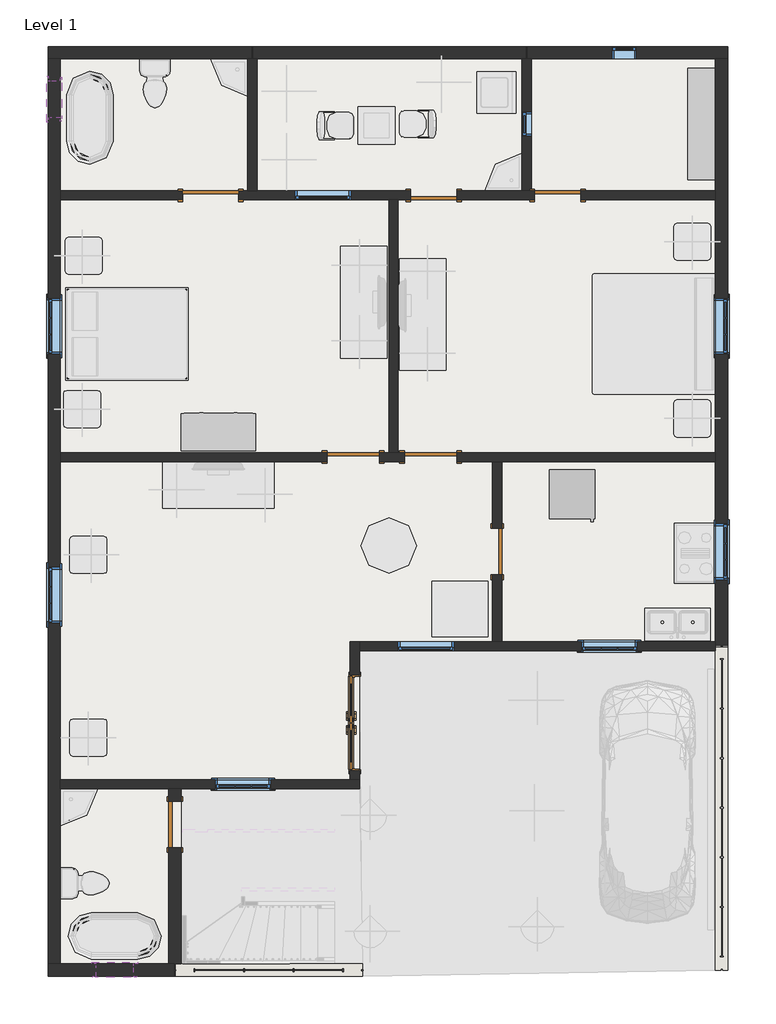
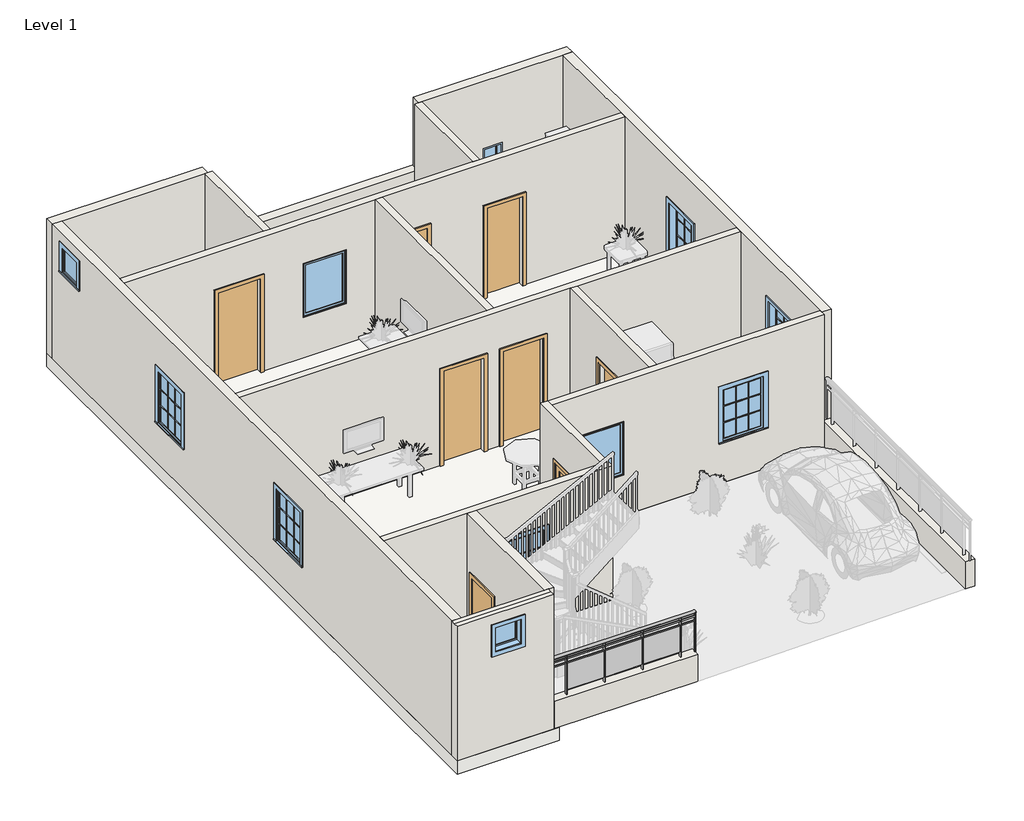
# One storey, part 1 of 3: 18 walls, 12 windows, 8 doors, 1 railing, 1 slab.
"""IFC4 building model written with IfcOpenShell, lengths in millimetres."""

from ifc_helpers import new_model, si_unit, point, frame, origin, origin_with_axes, place, context, project, spatial, polyline, ellipse_curve, trimmed, outline, extrude, faceted_brep, transform, mapped, element, save
from ifc_brep_helpers import plane_surface, extruded_surface, advanced_brep
from components import door_94998e6c, door_059fdd7e, door_255cab33, door_d8ec59b1, door_b6e9fca3, door_99d96fc5, door_16372e1c, window_29c06734, window_5c190c7e, window_7ecdf1d7, window_085f26e1, window_d657a5cb, window_e41d21a6

model = new_model("IFC4")

# Units and contexts
model_context = context("Model", 3, world=origin())
ifc_project = project(units=[si_unit("LENGTHUNIT", "METRE", prefix="MILLI")], contexts=[model_context])

# Site, building, storey
site = spatial("IfcSite", under=ifc_project)
building = spatial("IfcBuilding", under=site)
storey = spatial("IfcBuildingStorey", under=building, Name="Level 1", Elevation=0.0)

# Doors
placement = place(None, origin())
door_shape = door_94998e6c(model_context)
element("IfcDoor", 1, ObjectType="Door-Exterior-Double-Full Glass-Wood_Clad : 60\" x 80\"", at=placement, inside=storey, context=model_context, shape_type="MappedRepresentation", body=[
    mapped(door_shape, transform((-7732.5242777, 3282.853629, 0.0), x_axis=(0.0, 1.0, 0.0), y_axis=(-1.0, 0.0, 0.0), z_axis=(0.0, 0.0, 1.0))),
])
door_2_shape = door_059fdd7e(model_context)
element("IfcDoor", 2, ObjectType="Single-Flush : 30\" x 80\"", at=placement, inside=storey, context=model_context, shape_type="MappedRepresentation", body=[
    mapped(door_2_shape, transform((-6433.9492777, 11931.553629, 0.0), x_axis=(-1.0, 0.0, 0.0), y_axis=(0.0, -1.0, 0.0), z_axis=(0.0, 0.0, 1.0))),
])
element("IfcDoor", 3, ObjectType="Single-Flush : 30\" x 80\"", at=placement, inside=storey, context=model_context, shape_type="MappedRepresentation", body=[
    mapped(door_2_shape, transform((-5392.5492777, 6089.553629, 0.0), x_axis=(0.0, -1.0, 0.0), y_axis=(1.0, 0.0, 0.0), z_axis=(0.0, 0.0, 1.0))),
])
door_3_shape = door_255cab33(model_context)
element("IfcDoor", 4, ObjectType="Single-Flush : 30\" x 80\"", at=placement, inside=storey, context=model_context, shape_type="MappedRepresentation", body=[
    mapped(door_3_shape, transform((-4401.9492777, 11931.553629, 0.0), x_axis=(-1.0, 0.0, 0.0), y_axis=(0.0, -1.0, 0.0), z_axis=(0.0, 0.0, 1.0))),
])
door_4_shape = door_d8ec59b1(model_context)
element("IfcDoor", 5, ObjectType="Single-Flush : 30\" x 80\" 2", at=placement, inside=storey, context=model_context, shape_type="MappedRepresentation", body=[
    mapped(door_4_shape, transform((-10675.7492777, 1619.153629, 0.0), x_axis=(0.0, 1.0, 0.0), y_axis=(-1.0, 0.0, 0.0), z_axis=(0.0, 0.0, 1.0))),
])
door_5_shape = door_b6e9fca3(model_context)
element("IfcDoor", 6, ObjectType="Single-Flush : 34\" x 84\"", at=placement, inside=storey, context=model_context, shape_type="MappedRepresentation", body=[
    mapped(door_5_shape, transform((-7754.7492777, 7638.953629, 0.0), x_axis=(1.0, 0.0, 0.0), y_axis=(0.0, 1.0, 0.0), z_axis=(0.0, 0.0, 1.0))),
])
door_6_shape = door_99d96fc5(model_context)
element("IfcDoor", 7, ObjectType="Single-Flush : 34\" x 84\"", at=placement, inside=storey, context=model_context, shape_type="MappedRepresentation", body=[
    mapped(door_6_shape, transform((-6484.7492777, 7638.953629, 0.0), x_axis=(-1.0, 0.0, 0.0), y_axis=(0.0, -1.0, 0.0), z_axis=(0.0, 0.0, 1.0))),
])
door_7_shape = door_16372e1c(model_context)
element("IfcDoor", 8, ObjectType="Single-Flush : 36\" x 84\"", at=placement, inside=storey, context=model_context, shape_type="MappedRepresentation", body=[
    mapped(door_7_shape, transform((-10091.5492777, 11931.553629, 0.0), x_axis=(1.0, 0.0, 0.0), y_axis=(0.0, 1.0, 0.0), z_axis=(0.0, 0.0, 1.0))),
])

# Railing
element("IfcRailing", 9, ObjectType="Glass Panel - Bottom Fill", at=placement, inside=storey, context=model_context, shape_type="SolidModel", body=[
    advanced_brep(
    [(-10675.7492777, -730.346371, 1524.0), (-10675.7492777, -806.546371, 1524.0), (-7602.3492777, -730.346371, 1524.0), (-7602.3492777, -806.546371, 1524.0)],
    [
        (0, 1, ellipse_curve(frame((-10675.7492777, -768.446371, 1524.0), z_axis=(-1.0, 0.0, 0.0), x_axis=(0.0, -1.0, 0.0)), 38.1, 28.575)),
        (1, 0, ellipse_curve(frame((-10675.7492777, -768.446371, 1524.0), z_axis=(-1.0, 0.0, 0.0), x_axis=(0.0, -1.0, 0.0)), 38.1, 28.575)),
        (2, 3, ellipse_curve(frame((-7602.3492777, -768.446371, 1524.0), z_axis=(1.0, 0.0, 0.0), x_axis=(0.0, -1.0, 0.0)), 38.1, 28.575)),
        (3, 2, ellipse_curve(frame((-7602.3492777, -768.446371, 1524.0), z_axis=(1.0, 0.0, 0.0), x_axis=(0.0, -1.0, 0.0)), 38.1, 28.575)),
        (0, 2),
        (3, 1),
    ],
    [
        plane_surface(frame((-10675.7492777, -768.446371, 1524.0), z_axis=(-1.0, 0.0, 0.0), x_axis=(0.0, 1.0, 0.0))),
        plane_surface(frame((-7602.3492777, -768.446371, 1524.0), z_axis=(1.0, 0.0, 0.0), x_axis=(0.0, 1.0, 0.0))),
        extruded_surface(trimmed(ellipse_curve(frame((-7602.3492777, -768.446371, 1524.0), z_axis=(-1.0, 0.0, 0.0), x_axis=(0.0, -1.0, 0.0)), 38.1, 28.575), [point((-7602.3492777, -730.346371, 1524.0))], [point((-7602.3492777, -806.546371, 1524.0))], True, "CARTESIAN"), (-3073.4000000000005, 0.0, 0.0), 3073.4000000000005),
        extruded_surface(trimmed(ellipse_curve(frame((-7602.3492777, -768.446371, 1524.0), z_axis=(-1.0, 0.0, 0.0), x_axis=(0.0, -1.0, 0.0)), 38.1, 28.575), [point((-7602.3492777, -806.546371, 1524.0))], [point((-7602.3492777, -730.346371, 1524.0))], True, "CARTESIAN"), (-3073.4000000000005, 0.0, 0.0), 3073.4000000000005),
    ],
    [
        (0, [[1, 2]]),
        (1, [[3, 4]]),
        (2, [[-1, 5, -4, 6]]),
        (3, [[-2, -6, -3, -5]]),
    ],
),
    extrude(outline(polyline([(-10675.7492777, -781.146371), (-10675.7492777, -755.746371), (-7602.3492777, -755.746371), (-7602.3492777, -781.146371), (-10675.7492777, -781.146371)])), frame((0.0, 0.0, 1409.7), z_axis=(0.0, 0.0, 1.0), x_axis=(1.0, 0.0, 0.0)), (0.0, 0.0, 1.0), 25.4),
    extrude(outline(polyline([(-10675.7492777, -781.146371), (-10675.7492777, -755.746371), (-7602.3492777, -755.746371), (-7602.3492777, -781.146371), (-10675.7492777, -781.146371)])), frame((0.0, 0.0, 1308.1), z_axis=(0.0, 0.0, 1.0), x_axis=(1.0, 0.0, 0.0)), (0.0, 0.0, 1.0), 25.4),
    extrude(outline(polyline([(-7926.1992777, -793.846371), (-7926.1992777, -743.046371), (-7913.4992777, -743.046371), (-7913.4992777, -793.846371), (-7926.1992777, -793.846371)])), frame((0.0, 0.0, 609.6), z_axis=(0.0, 0.0, 1.0), x_axis=(1.0, 0.0, 0.0)), (0.0, 0.0, 1.0), 885.6788223),
    extrude(outline(polyline([(-8732.6492777, -761.911214), (-7919.8492777, -761.911214), (-7919.8492777, -768.261214), (-8732.6492777, -768.261214), (-8732.6492777, -761.911214)])), frame((0.0, 0.0, 711.2), z_axis=(0.0, 0.0, 1.0), x_axis=(1.0, 0.0, 0.0)), (0.0, 0.0, 1.0), 596.9),
    extrude(outline(polyline([(-8738.9992777, -793.846371), (-8738.9992777, -743.046371), (-8726.2992777, -743.046371), (-8726.2992777, -793.846371), (-8738.9992777, -793.846371)])), frame((0.0, 0.0, 609.6), z_axis=(0.0, 0.0, 1.0), x_axis=(1.0, 0.0, 0.0)), (0.0, 0.0, 1.0), 885.6788223),
    extrude(outline(polyline([(-9545.4492777, -761.911214), (-8732.6492777, -761.911214), (-8732.6492777, -768.261214), (-9545.4492777, -768.261214), (-9545.4492777, -761.911214)])), frame((0.0, 0.0, 711.2), z_axis=(0.0, 0.0, 1.0), x_axis=(1.0, 0.0, 0.0)), (0.0, 0.0, 1.0), 596.9),
    extrude(outline(polyline([(-9551.7992777, -793.846371), (-9551.7992777, -743.046371), (-9539.0992777, -743.046371), (-9539.0992777, -793.846371), (-9551.7992777, -793.846371)])), frame((0.0, 0.0, 609.6), z_axis=(0.0, 0.0, 1.0), x_axis=(1.0, 0.0, 0.0)), (0.0, 0.0, 1.0), 885.6788223),
    extrude(outline(polyline([(-10358.2492777, -761.911214), (-9545.4492777, -761.911214), (-9545.4492777, -768.261214), (-10358.2492777, -768.261214), (-10358.2492777, -761.911214)])), frame((0.0, 0.0, 711.2), z_axis=(0.0, 0.0, 1.0), x_axis=(1.0, 0.0, 0.0)), (0.0, 0.0, 1.0), 596.9),
    extrude(outline(polyline([(-10364.5992777, -793.846371), (-10364.5992777, -743.046371), (-10351.8992777, -743.046371), (-10351.8992777, -793.846371), (-10364.5992777, -793.846371)])), frame((0.0, 0.0, 609.6), z_axis=(0.0, 0.0, 1.0), x_axis=(1.0, 0.0, 0.0)), (0.0, 0.0, 1.0), 885.6788223),
    extrude(outline(polyline([(-7615.0492777, -777.971371), (-7615.0492777, -758.921371), (-7595.9992777, -758.921371), (-7595.9992777, -777.971371), (-7615.0492777, -777.971371)])), frame((0.0, 0.0, 609.6), z_axis=(0.0, 0.0, 1.0), x_axis=(1.0, 0.0, 0.0)), (0.0, 0.0, 1.0), 885.6788223),
    extrude(outline(polyline([(-10682.0992777, -777.971371), (-10682.0992777, -758.921371), (-10663.0492777, -758.921371), (-10663.0492777, -777.971371), (-10682.0992777, -777.971371)])), frame((0.0, 0.0, 609.6), z_axis=(0.0, 0.0, 1.0), x_axis=(1.0, 0.0, 0.0)), (0.0, 0.0, 1.0), 885.6788223),
])

# Slab
element("IfcSlab", 10, ObjectType="Generic - 12\"", at=placement, inside=storey, context=model_context, shape_type="SweptSolid", body=[
    extrude(outline(polyline([(-1607.9492777, 14369.953629), (-1607.9492777, 4463.953629), (-7653.1492777, 4463.953629), (-7653.1492777, 2203.353629), (-10574.1492777, 2203.353629), (-10574.1492777, -870.046371), (-12758.5492777, -870.046371), (-12758.5492777, 14369.953629), (-1607.9492777, 14369.953629)])), frame((0.0, 0.0, -304.8), z_axis=(0.0, 0.0, 1.0), x_axis=(1.0, 0.0, 0.0)), (0.0, 0.0, 1.0), 304.8),
])

# Walls
element("IfcWall", 11, ObjectType="Generic - 2'", at=placement, inside=storey, context=model_context, shape_type="Brep", body=[
    faceted_brep([(-1811.1492777, 4527.453629, 0.0), (-1811.1492777, 4463.953629, 0.0), (-1811.1492777, -768.446371, 0.0), (-1811.1492777, -768.446371, 609.6), (-1811.1492777, 4527.453629, 609.6), (-1607.9492777, 4527.453629, 0.0), (-1607.9492777, 4527.453629, 609.6), (-1607.9492777, -768.446371, 609.6), (-1607.9492777, -768.446371, 0.0)], [[[0, 1, 2, 3, 4]], [[5, 6, 7, 8]], [[2, 1, 0, 5, 8]], [[3, 2, 8, 7]], [[4, 3, 7, 6]], [[0, 4, 6, 5]]]),
])
element("IfcWall", 12, ObjectType="Generic - 2'", at=placement, inside=storey, context=model_context, shape_type="SweptSolid", body=[
    extrude(outline(polyline([(-10663.0492777, -666.846371), (-7602.3492777, -666.846371), (-7602.3492777, -870.046371), (-10663.0492777, -870.046371), (-10663.0492777, -666.846371)])), origin_with_axes(), (0.0, 0.0, 1.0), 609.6),
])
element("IfcWall", 13, ObjectType="Generic - 8\"", at=placement, inside=storey, context=model_context, shape_type="Brep", body=[
    faceted_brep([(-12758.5492777, 14166.753629, 0.0), (-12555.3492777, 14166.753629, 0.0), (-9418.4492777, 14166.753629, 0.0), (-9418.4492777, 14166.753629, 3048.0), (-12555.3492777, 14166.753629, 3048.0), (-12758.5492777, 14166.753629, 3048.0), (-12758.5492777, 14369.953629, 0.0), (-12758.5492777, 14369.953629, 3048.0), (-9418.4492777, 14369.953629, 3048.0), (-9418.4492777, 14369.953629, 0.0)], [[[0, 1, 2, 3, 4, 5]], [[6, 7, 8, 9]], [[2, 1, 0, 6, 9]], [[3, 2, 9, 8]], [[0, 5, 7, 6]], [[5, 4, 3, 8, 7]]]),
])
element("IfcWall", 14, ObjectType="Generic - 8\"", at=placement, inside=storey, context=model_context, shape_type="Brep", body=[
    faceted_brep([(-1811.1492777, 14166.753629, 0.0), (-1811.1492777, 12007.753629, 0.0), (-1811.1492777, 11855.353629, 0.0), (-1811.1492777, 7715.153629, 0.0), (-1811.1492777, 7562.753629, 0.0), (-1811.1492777, 4552.853629, 0.0), (-1811.1492777, 4552.853629, 3048.0), (-1811.1492777, 7562.753629, 3048.0), (-1811.1492777, 7715.153629, 3048.0), (-1811.1492777, 11855.353629, 3048.0), (-1811.1492777, 12007.753629, 3048.0), (-1811.1492777, 14166.753629, 3048.0), (-1811.1492777, 9328.053629, 2133.6), (-1811.1492777, 9328.053629, 914.4), (-1811.1492777, 10242.453629, 914.4), (-1811.1492777, 10242.453629, 2133.6), (-1811.1492777, 5632.353629, 2133.6), (-1811.1492777, 5632.353629, 914.4), (-1811.1492777, 6546.753629, 914.4), (-1811.1492777, 6546.753629, 2133.6), (-1607.9492777, 14166.753629, 0.0), (-1607.9492777, 14166.753629, 3048.0), (-1607.9492777, 4552.853629, 3048.0), (-1607.9492777, 4552.853629, 0.0), (-1607.9492777, 9328.053629, 2133.6), (-1607.9492777, 10242.453629, 2133.6), (-1607.9492777, 10242.453629, 914.4), (-1607.9492777, 9328.053629, 914.4), (-1607.9492777, 5632.353629, 2133.6), (-1607.9492777, 6546.753629, 2133.6), (-1607.9492777, 6546.753629, 914.4), (-1607.9492777, 5632.353629, 914.4)], [[[0, 1, 2, 3, 4, 5, 6, 7, 8, 9, 10, 11], [12, 13, 14, 15], [16, 17, 18, 19]], [[20, 21, 22, 23], [24, 25, 26, 27], [28, 29, 30, 31]], [[5, 4, 3, 2, 1, 0, 20, 23]], [[6, 5, 23, 22]], [[0, 11, 21, 20]], [[13, 12, 24, 27]], [[14, 13, 27, 26]], [[15, 14, 26, 25]], [[12, 15, 25, 24]], [[17, 16, 28, 31]], [[18, 17, 31, 30]], [[19, 18, 30, 29]], [[16, 19, 29, 28]], [[11, 10, 9, 8, 7, 6, 22, 21]]]),
])
element("IfcWall", 15, ObjectType="Generic - 8\"", at=placement, inside=storey, context=model_context, shape_type="Brep", body=[
    faceted_brep([(-12555.3492777, -666.846371, 0.0), (-12555.3492777, 2203.353629, 0.0), (-12555.3492777, 2355.753629, 0.0), (-12555.3492777, 7562.753629, 0.0), (-12555.3492777, 7715.153629, 0.0), (-12555.3492777, 11855.353629, 0.0), (-12555.3492777, 12007.753629, 0.0), (-12555.3492777, 14166.753629, 0.0), (-12555.3492777, 14166.753629, 3048.0), (-12555.3492777, 12007.753629, 3048.0), (-12555.3492777, 11855.353629, 3048.0), (-12555.3492777, 7715.153629, 3048.0), (-12555.3492777, 7562.753629, 3048.0), (-12555.3492777, 2355.753629, 3048.0), (-12555.3492777, 2203.353629, 3048.0), (-12555.3492777, -666.846371, 3048.0), (-12555.3492777, 13811.153629, 2768.6), (-12555.3492777, 13811.153629, 2159.0), (-12555.3492777, 13201.553629, 2159.0), (-12555.3492777, 13201.553629, 2768.6), (-12555.3492777, 10242.453629, 2133.6), (-12555.3492777, 10242.453629, 914.4), (-12555.3492777, 9328.053629, 914.4), (-12555.3492777, 9328.053629, 2133.6), (-12555.3492777, 5835.553629, 2133.6), (-12555.3492777, 5835.553629, 914.4), (-12555.3492777, 4921.153629, 914.4), (-12555.3492777, 4921.153629, 2133.6), (-12758.5492777, -666.846371, 0.0), (-12758.5492777, -666.846371, 3048.0), (-12758.5492777, 14166.753629, 3048.0), (-12758.5492777, 14166.753629, 0.0), (-12758.5492777, 13811.153629, 2768.6), (-12758.5492777, 13201.553629, 2768.6), (-12758.5492777, 13201.553629, 2159.0), (-12758.5492777, 13811.153629, 2159.0), (-12758.5492777, 10242.453629, 2133.6), (-12758.5492777, 9328.053629, 2133.6), (-12758.5492777, 9328.053629, 914.4), (-12758.5492777, 10242.453629, 914.4), (-12758.5492777, 5835.553629, 2133.6), (-12758.5492777, 4921.153629, 2133.6), (-12758.5492777, 4921.153629, 914.4), (-12758.5492777, 5835.553629, 914.4)], [[[0, 1, 2, 3, 4, 5, 6, 7, 8, 9, 10, 11, 12, 13, 14, 15], [16, 17, 18, 19], [20, 21, 22, 23], [24, 25, 26, 27]], [[28, 29, 30, 31], [32, 33, 34, 35], [36, 37, 38, 39], [40, 41, 42, 43]], [[7, 6, 5, 4, 3, 2, 1, 0, 28, 31]], [[8, 7, 31, 30]], [[0, 15, 29, 28]], [[17, 16, 32, 35]], [[18, 17, 35, 34]], [[19, 18, 34, 33]], [[16, 19, 33, 32]], [[21, 20, 36, 39]], [[22, 21, 39, 38]], [[23, 22, 38, 37]], [[20, 23, 37, 36]], [[25, 24, 40, 43]], [[26, 25, 43, 42]], [[27, 26, 42, 41]], [[24, 27, 41, 40]], [[15, 14, 13, 12, 11, 10, 9, 8, 30, 29]]]),
])
element("IfcWall", 16, ObjectType="Generic - 8\"", at=placement, inside=storey, context=model_context, shape_type="Brep", body=[
    faceted_brep([(-10777.3492777, -666.846371, 0.0), (-10777.3492777, -666.846371, 3048.0), (-10777.3492777, 2203.353629, 3048.0), (-10777.3492777, 2203.353629, 0.0), (-10777.3492777, 2000.153629, 0.0), (-10777.3492777, 2000.153629, 1727.2), (-10777.3492777, 1238.153629, 1727.2), (-10777.3492777, 1238.153629, 0.0), (-10574.1492777, -666.846371, 3048.0), (-10574.1492777, -666.846371, 0.0), (-10574.1492777, 1238.153629, 0.0), (-10574.1492777, 1238.153629, 1727.2), (-10574.1492777, 2000.153629, 1727.2), (-10574.1492777, 2000.153629, 0.0), (-10574.1492777, 2203.353629, 0.0), (-10574.1492777, 2203.353629, 3048.0), (-10688.4492777, -666.846371, 0.0), (-10688.4492777, -666.846371, 3048.0)], [[[0, 1, 2, 3, 4, 5, 6, 7]], [[8, 9, 10, 11, 12, 13, 14, 15]], [[3, 14, 13, 4]], [[9, 16, 0, 7, 10]], [[1, 0, 16, 9, 8, 17]], [[3, 2, 15, 14]], [[5, 12, 11, 6]], [[6, 11, 10, 7]], [[12, 5, 4, 13]], [[2, 1, 17, 8, 15]]]),
])
element("IfcWall", 17, ObjectType="Generic - 8\"", at=placement, inside=storey, context=model_context, shape_type="Brep", body=[
    faceted_brep([(-4897.2492777, 14166.753629, 0.0), (-4833.7492777, 14166.753629, 0.0), (-1811.1492777, 14166.753629, 0.0), (-1607.9492777, 14166.753629, 0.0), (-1607.9492777, 14166.753629, 3048.0), (-1811.1492777, 14166.753629, 3048.0), (-4833.7492777, 14166.753629, 3048.0), (-4897.2492777, 14166.753629, 3048.0), (-3106.5492777, 14166.753629, 1524.0), (-3106.5492777, 14166.753629, 914.4), (-3512.9492777, 14166.753629, 914.4), (-3512.9492777, 14166.753629, 1524.0), (-4897.2492777, 14369.953629, 0.0), (-4897.2492777, 14369.953629, 3048.0), (-1607.9492777, 14369.953629, 3048.0), (-1607.9492777, 14369.953629, 0.0), (-3106.5492777, 14369.953629, 1524.0), (-3512.9492777, 14369.953629, 1524.0), (-3512.9492777, 14369.953629, 914.4), (-3106.5492777, 14369.953629, 914.4)], [[[0, 1, 2, 3, 4, 5, 6, 7], [8, 9, 10, 11]], [[12, 13, 14, 15], [16, 17, 18, 19]], [[3, 2, 1, 0, 12, 15]], [[0, 7, 13, 12]], [[4, 3, 15, 14]], [[9, 8, 16, 19]], [[10, 9, 19, 18]], [[11, 10, 18, 17]], [[8, 11, 17, 16]], [[7, 6, 5, 4, 14, 13]]]),
])
element("IfcWall", 18, ObjectType="Generic - 8\"", at=placement, inside=storey, context=model_context, shape_type="Brep", body=[
    faceted_brep([(-9393.0492777, 14166.753629, 0.0), (-9329.5492777, 14166.753629, 0.0), (-4922.6492777, 14166.753629, 0.0), (-4922.6492777, 14166.753629, 1524.0), (-9393.0492777, 14166.753629, 1524.0), (-9393.0492777, 14369.953629, 0.0), (-9393.0492777, 14369.953629, 1524.0), (-4922.6492777, 14369.953629, 1524.0), (-4922.6492777, 14369.953629, 0.0)], [[[0, 1, 2, 3, 4]], [[5, 6, 7, 8]], [[2, 1, 0, 5, 8]], [[3, 2, 8, 7]], [[4, 3, 7, 6]], [[0, 4, 6, 5]]]),
])
element("IfcWall", 19, ObjectType="Generic - 8\"", at=placement, inside=storey, context=model_context, shape_type="Brep", body=[
    faceted_brep([(-10688.4492777, -666.846371, 0.0), (-10777.3492777, -666.846371, 0.0), (-12555.3492777, -666.846371, 0.0), (-12758.5492777, -666.846371, 0.0), (-12758.5492777, -666.846371, 3048.0), (-12555.3492777, -666.846371, 3048.0), (-10777.3492777, -666.846371, 3048.0), (-10688.4492777, -666.846371, 3048.0), (-11361.5492777, -666.846371, 2768.6), (-11971.1492777, -666.846371, 2768.6), (-11971.1492777, -666.846371, 2159.0), (-11361.5492777, -666.846371, 2159.0), (-10688.4492777, -870.046371, 0.0), (-10688.4492777, -870.046371, 3048.0), (-12758.5492777, -870.046371, 3048.0), (-12758.5492777, -870.046371, 0.0), (-11361.5492777, -870.046371, 2768.6), (-11361.5492777, -870.046371, 2159.0), (-11971.1492777, -870.046371, 2159.0), (-11971.1492777, -870.046371, 2768.6), (-10688.4492777, -768.446371, 3048.0), (-12758.5492777, -768.446371, 3048.0)], [[[0, 1, 2, 3, 4, 5, 6, 7], [8, 9, 10, 11]], [[12, 13, 14, 15], [16, 17, 18, 19]], [[3, 2, 1, 0, 12, 15]], [[0, 7, 20, 13, 12]], [[4, 3, 15, 14, 21]], [[16, 19, 9, 8]], [[19, 18, 10, 9]], [[18, 17, 11, 10]], [[17, 16, 8, 11]], [[21, 14, 13, 20]], [[7, 6, 5, 4, 21, 20]]]),
])
element("IfcWall", 20, ObjectType="INNER 6'", at=placement, inside=storey, context=model_context, shape_type="Brep", body=[
    faceted_brep([(-6052.9492777, 11855.353629, 0.0), (-4782.9492777, 11855.353629, 0.0), (-4782.9492777, 11855.353629, 2032.0), (-4020.9492777, 11855.353629, 2032.0), (-4020.9492777, 11855.353629, 0.0), (-1811.1492777, 11855.353629, 0.0), (-1811.1492777, 11855.353629, 3048.0), (-7018.1492777, 11855.353629, 3048.0), (-7170.5492777, 11855.353629, 3048.0), (-12555.3492777, 11855.353629, 3048.0), (-12555.3492777, 11855.353629, 0.0), (-10548.7492777, 11855.353629, 0.0), (-10548.7492777, 11855.353629, 2133.6), (-9634.3492777, 11855.353629, 2133.6), (-9634.3492777, 11855.353629, 0.0), (-7170.5492777, 11855.353629, 0.0), (-7018.1492777, 11855.353629, 0.0), (-6814.9492777, 11855.353629, 0.0), (-6814.9492777, 11855.353629, 2032.0), (-6052.9492777, 11855.353629, 2032.0), (-8707.2492777, 11855.353629, 2133.6), (-7792.8492777, 11855.353629, 2133.6), (-7792.8492777, 11855.353629, 914.4), (-8707.2492777, 11855.353629, 914.4), (-4782.9492777, 12007.753629, 2032.0), (-4782.9492777, 12007.753629, 0.0), (-4833.7492777, 12007.753629, 0.0), (-4986.1492777, 12007.753629, 0.0), (-6052.9492777, 12007.753629, 0.0), (-6052.9492777, 12007.753629, 2032.0), (-6814.9492777, 12007.753629, 2032.0), (-6814.9492777, 12007.753629, 0.0), (-9329.5492777, 12007.753629, 0.0), (-9481.9492777, 12007.753629, 0.0), (-9634.3492777, 12007.753629, 0.0), (-9634.3492777, 12007.753629, 2133.6), (-10548.7492777, 12007.753629, 2133.6), (-10548.7492777, 12007.753629, 0.0), (-12555.3492777, 12007.753629, 0.0), (-12555.3492777, 12007.753629, 3048.0), (-9481.9492777, 12007.753629, 3048.0), (-9329.5492777, 12007.753629, 3048.0), (-4986.1492777, 12007.753629, 3048.0), (-4833.7492777, 12007.753629, 3048.0), (-1811.1492777, 12007.753629, 3048.0), (-1811.1492777, 12007.753629, 0.0), (-4020.9492777, 12007.753629, 0.0), (-4020.9492777, 12007.753629, 2032.0), (-8707.2492777, 12007.753629, 2133.6), (-8707.2492777, 12007.753629, 914.4), (-7792.8492777, 12007.753629, 914.4), (-7792.8492777, 12007.753629, 2133.6)], [[[0, 1, 2, 3, 4, 5, 6, 7, 8, 9, 10, 11, 12, 13, 14, 15, 16, 17, 18, 19], [20, 21, 22, 23]], [[24, 25, 26, 27, 28, 29, 30, 31, 32, 33, 34, 35, 36, 37, 38, 39, 40, 41, 42, 43, 44, 45, 46, 47], [48, 49, 50, 51]], [[11, 10, 38, 37]], [[34, 33, 32, 31, 17, 16, 15, 14]], [[46, 45, 5, 4]], [[28, 27, 26, 25, 1, 0]], [[6, 5, 45, 44]], [[10, 9, 39, 38]], [[35, 34, 14, 13]], [[36, 35, 13, 12]], [[37, 36, 12, 11]], [[18, 17, 31, 30]], [[19, 18, 30, 29]], [[0, 19, 29, 28]], [[2, 1, 25, 24]], [[3, 2, 24, 47]], [[4, 3, 47, 46]], [[49, 48, 20, 23]], [[50, 49, 23, 22]], [[51, 50, 22, 21]], [[48, 51, 21, 20]], [[9, 8, 7, 6, 44, 43, 42, 41, 40, 39]]]),
])
element("IfcWall", 21, ObjectType="INNER 6'", at=placement, inside=storey, context=model_context, shape_type="SweptSolid", body=[
    extrude(outline(polyline([(-7170.5492777, 7715.153629), (-7170.5492777, 11855.353629), (-7018.1492777, 11855.353629), (-7018.1492777, 7715.153629), (-7170.5492777, 7715.153629)])), origin_with_axes(), (0.0, 0.0, 1.0), 3048.0),
])
element("IfcWall", 22, ObjectType="INNER 6'", at=placement, inside=storey, context=model_context, shape_type="Brep", body=[
    faceted_brep([(-6916.5492777, 7715.153629, 2133.6), (-6916.5492777, 7715.153629, 0.0), (-7018.1492777, 7715.153629, 0.0), (-7170.5492777, 7715.153629, 0.0), (-7322.9492777, 7715.153629, 0.0), (-7322.9492777, 7715.153629, 2133.6), (-8186.5492777, 7715.153629, 2133.6), (-8186.5492777, 7715.153629, 0.0), (-12555.3492777, 7715.153629, 0.0), (-12555.3492777, 7715.153629, 3048.0), (-7170.5492777, 7715.153629, 3048.0), (-7018.1492777, 7715.153629, 3048.0), (-1811.1492777, 7715.153629, 3048.0), (-1811.1492777, 7715.153629, 0.0), (-6052.9492777, 7715.153629, 0.0), (-6052.9492777, 7715.153629, 2133.6), (-7322.9492777, 7562.753629, 0.0), (-6916.5492777, 7562.753629, 0.0), (-6916.5492777, 7562.753629, 2133.6), (-6052.9492777, 7562.753629, 2133.6), (-6052.9492777, 7562.753629, 0.0), (-5468.7492777, 7562.753629, 0.0), (-5316.3492777, 7562.753629, 0.0), (-1811.1492777, 7562.753629, 0.0), (-1811.1492777, 7562.753629, 3048.0), (-5316.3492777, 7562.753629, 3048.0), (-5468.7492777, 7562.753629, 3048.0), (-12555.3492777, 7562.753629, 3048.0), (-12555.3492777, 7562.753629, 0.0), (-8186.5492777, 7562.753629, 0.0), (-8186.5492777, 7562.753629, 2133.6), (-7322.9492777, 7562.753629, 2133.6)], [[[0, 1, 2, 3, 4, 5, 6, 7, 8, 9, 10, 11, 12, 13, 14, 15]], [[16, 17, 18, 19, 20, 21, 22, 23, 24, 25, 26, 27, 28, 29, 30, 31]], [[29, 28, 8, 7]], [[14, 13, 23, 22, 21, 20]], [[4, 3, 2, 1, 17, 16]], [[9, 8, 28, 27]], [[13, 12, 24, 23]], [[5, 4, 16, 31]], [[6, 5, 31, 30]], [[7, 6, 30, 29]], [[18, 17, 1, 0]], [[19, 18, 0, 15]], [[20, 19, 15, 14]], [[12, 11, 10, 9, 27, 26, 25, 24]]]),
])
element("IfcWall", 23, ObjectType="INNER 6'", at=placement, inside=storey, context=model_context, shape_type="Brep", body=[
    faceted_brep([(-12555.3492777, 2203.353629, 0.0), (-10777.3492777, 2203.353629, 0.0), (-10574.1492777, 2203.353629, 0.0), (-7653.1492777, 2203.353629, 0.0), (-7653.1492777, 2203.353629, 3048.0), (-10574.1492777, 2203.353629, 3048.0), (-10777.3492777, 2203.353629, 3048.0), (-12555.3492777, 2203.353629, 3048.0), (-10015.3492777, 2203.353629, 2133.6), (-9100.9492777, 2203.353629, 2133.6), (-9100.9492777, 2203.353629, 914.4), (-10015.3492777, 2203.353629, 914.4), (-12555.3492777, 2355.753629, 0.0), (-12555.3492777, 2355.753629, 3048.0), (-7805.5492777, 2355.753629, 3048.0), (-7653.1492777, 2355.753629, 3048.0), (-7653.1492777, 2355.753629, 0.0), (-7805.5492777, 2355.753629, 0.0), (-10015.3492777, 2355.753629, 2133.6), (-10015.3492777, 2355.753629, 914.4), (-9100.9492777, 2355.753629, 914.4), (-9100.9492777, 2355.753629, 2133.6)], [[[0, 1, 2, 3, 4, 5, 6, 7], [8, 9, 10, 11]], [[12, 13, 14, 15, 16, 17], [18, 19, 20, 21]], [[3, 2, 1, 0, 12, 17, 16]], [[0, 7, 13, 12]], [[4, 3, 16, 15]], [[19, 18, 8, 11]], [[20, 19, 11, 10]], [[21, 20, 10, 9]], [[18, 21, 9, 8]], [[7, 6, 5, 4, 15, 14, 13]]]),
])
element("IfcWall", 24, ObjectType="INNER 6'", at=placement, inside=storey, context=model_context, shape_type="Brep", body=[
    faceted_brep([(-7653.1492777, 2355.753629, 3048.0), (-7653.1492777, 2355.753629, 0.0), (-7653.1492777, 2495.453629, 0.0), (-7653.1492777, 2495.453629, 2057.4), (-7653.1492777, 4070.253629, 2057.4), (-7653.1492777, 4070.253629, 0.0), (-7653.1492777, 4463.953629, 0.0), (-7653.1492777, 4616.353629, 0.0), (-7653.1492777, 4616.353629, 3048.0), (-7653.1492777, 4463.953629, 3048.0), (-7805.5492777, 2355.753629, 0.0), (-7805.5492777, 2355.753629, 3048.0), (-7805.5492777, 4616.353629, 3048.0), (-7805.5492777, 4616.353629, 0.0), (-7805.5492777, 4070.253629, 0.0), (-7805.5492777, 4070.253629, 2057.4), (-7805.5492777, 2495.453629, 2057.4), (-7805.5492777, 2495.453629, 0.0)], [[[0, 1, 2, 3, 4, 5, 6, 7, 8, 9]], [[10, 11, 12, 13, 14, 15, 16, 17]], [[1, 10, 17, 2]], [[13, 7, 6, 5, 14]], [[1, 0, 11, 10]], [[8, 7, 13, 12]], [[4, 15, 14, 5]], [[15, 4, 3, 16]], [[16, 3, 2, 17]], [[0, 9, 8, 12, 11]]]),
])
element("IfcWall", 25, ObjectType="INNER 6'", at=placement, inside=storey, context=model_context, shape_type="Brep", body=[
    faceted_brep([(-7653.1492777, 4463.953629, 0.0), (-1811.1492777, 4463.953629, 0.0), (-1811.1492777, 4463.953629, 3048.0), (-7653.1492777, 4463.953629, 3048.0), (-4008.2492777, 4463.953629, 2133.6), (-3093.8492777, 4463.953629, 2133.6), (-3093.8492777, 4463.953629, 914.4), (-4008.2492777, 4463.953629, 914.4), (-7018.1492777, 4463.953629, 2133.6), (-6103.7492777, 4463.953629, 2133.6), (-6103.7492777, 4463.953629, 914.4), (-7018.1492777, 4463.953629, 914.4), (-7653.1492777, 4616.353629, 0.0), (-7653.1492777, 4616.353629, 3048.0), (-5468.7492777, 4616.353629, 3048.0), (-5316.3492777, 4616.353629, 3048.0), (-1811.1492777, 4616.353629, 3048.0), (-1811.1492777, 4616.353629, 0.0), (-5316.3492777, 4616.353629, 0.0), (-5468.7492777, 4616.353629, 0.0), (-4008.2492777, 4616.353629, 2133.6), (-4008.2492777, 4616.353629, 914.4), (-3093.8492777, 4616.353629, 914.4), (-3093.8492777, 4616.353629, 2133.6), (-7018.1492777, 4616.353629, 2133.6), (-7018.1492777, 4616.353629, 914.4), (-6103.7492777, 4616.353629, 914.4), (-6103.7492777, 4616.353629, 2133.6), (-1811.1492777, 4527.453629, 0.0)], [[[0, 1, 2, 3], [4, 5, 6, 7], [8, 9, 10, 11]], [[12, 13, 14, 15, 16, 17, 18, 19], [20, 21, 22, 23], [24, 25, 26, 27]], [[1, 0, 12, 19, 18, 17, 28]], [[0, 3, 13, 12]], [[2, 1, 28, 17, 16]], [[21, 20, 4, 7]], [[22, 21, 7, 6]], [[23, 22, 6, 5]], [[20, 23, 5, 4]], [[25, 24, 8, 11]], [[26, 25, 11, 10]], [[27, 26, 10, 9]], [[24, 27, 9, 8]], [[3, 2, 16, 15, 14, 13]]]),
])
element("IfcWall", 26, ObjectType="INNER 6'", at=placement, inside=storey, context=model_context, shape_type="SweptSolid", body=[
    extrude(outline(polyline([(5708.553629, 2032.0), (5708.553629, 0.0), (4616.353629, 0.0), (4616.353629, 3048.0), (7562.753629, 3048.0), (7562.753629, 0.0), (6470.553629, 0.0), (6470.553629, 2032.0), (5708.553629, 2032.0)])), frame((-5468.7492777, 0.0, 0.0), z_axis=(1.0, 0.0, 0.0), x_axis=(0.0, 1.0, 0.0)), (0.0, 0.0, 1.0), 152.4),
])
element("IfcWall", 27, ObjectType="INNER 6'", at=placement, inside=storey, context=model_context, shape_type="Brep", body=[
    faceted_brep([(-9481.9492777, 14166.753629, 0.0), (-9481.9492777, 12007.753629, 0.0), (-9481.9492777, 12007.753629, 3048.0), (-9481.9492777, 14166.753629, 3048.0), (-9329.5492777, 14166.753629, 0.0), (-9329.5492777, 14166.753629, 3048.0), (-9329.5492777, 12007.753629, 3048.0), (-9329.5492777, 12007.753629, 0.0), (-9393.0492777, 14166.753629, 0.0)], [[[0, 1, 2, 3]], [[4, 5, 6, 7]], [[1, 0, 8, 4, 7]], [[0, 3, 5, 4, 8]], [[2, 1, 7, 6]], [[3, 2, 6, 5]]]),
])
element("IfcWall", 28, ObjectType="INNER 6'", at=placement, inside=storey, context=model_context, shape_type="Brep", body=[
    faceted_brep([(-4986.1492777, 14166.753629, 0.0), (-4986.1492777, 12007.753629, 0.0), (-4986.1492777, 12007.753629, 3048.0), (-4986.1492777, 14166.753629, 3048.0), (-4986.1492777, 13303.153629, 1524.0), (-4986.1492777, 12896.753629, 1524.0), (-4986.1492777, 12896.753629, 914.4), (-4986.1492777, 13303.153629, 914.4), (-4833.7492777, 14166.753629, 0.0), (-4833.7492777, 14166.753629, 3048.0), (-4833.7492777, 12007.753629, 3048.0), (-4833.7492777, 12007.753629, 0.0), (-4833.7492777, 13303.153629, 1524.0), (-4833.7492777, 13303.153629, 914.4), (-4833.7492777, 12896.753629, 914.4), (-4833.7492777, 12896.753629, 1524.0), (-4897.2492777, 14166.753629, 0.0), (-4897.2492777, 14166.753629, 3048.0)], [[[0, 1, 2, 3], [4, 5, 6, 7]], [[8, 9, 10, 11], [12, 13, 14, 15]], [[1, 0, 16, 8, 11]], [[0, 3, 17, 9, 8, 16]], [[2, 1, 11, 10]], [[13, 12, 4, 7]], [[14, 13, 7, 6]], [[15, 14, 6, 5]], [[12, 15, 5, 4]], [[3, 2, 10, 9, 17]]]),
])

# Windows
window_shape = window_29c06734(model_context)
element("IfcWindow", 29, ObjectType="Casement 3x3 with Trim : 36\" x 48\"", at=placement, inside=storey, context=model_context, shape_type="MappedRepresentation", body=[
    mapped(window_shape, transform((-12656.9492777, 9785.253629, 0.0), x_axis=(0.0, 1.0, 0.0), y_axis=(-1.0, 0.0, 0.0), z_axis=(0.0, 0.0, 1.0))),
])
element("IfcWindow", 30, ObjectType="Casement 3x3 with Trim : 36\" x 48\"", at=placement, inside=storey, context=model_context, shape_type="MappedRepresentation", body=[
    mapped(window_shape, transform((-1709.5492777, 9785.253629, 0.0), x_axis=(0.0, -1.0, 0.0), y_axis=(1.0, 0.0, 0.0), z_axis=(0.0, 0.0, 1.0))),
])
element("IfcWindow", 31, ObjectType="Casement 3x3 with Trim : 36\" x 48\"", at=placement, inside=storey, context=model_context, shape_type="MappedRepresentation", body=[
    mapped(window_shape, transform((-12656.9492777, 5378.353629, 0.0), x_axis=(0.0, 1.0, 0.0), y_axis=(-1.0, 0.0, 0.0), z_axis=(0.0, 0.0, 1.0))),
])
element("IfcWindow", 32, ObjectType="Casement 3x3 with Trim : 36\" x 48\"", at=placement, inside=storey, context=model_context, shape_type="MappedRepresentation", body=[
    mapped(window_shape, transform((-1709.5492777, 6089.553629, 0.0), x_axis=(0.0, -1.0, 0.0), y_axis=(1.0, 0.0, 0.0), z_axis=(0.0, 0.0, 1.0))),
])
window_2_shape = window_5c190c7e(model_context)
element("IfcWindow", 33, ObjectType="Casement 3x3 with Trim : 36\" x 48\"", at=placement, inside=storey, context=model_context, shape_type="MappedRepresentation", body=[
    mapped(window_2_shape, transform((-9558.1492777, 2279.553629, 0.0), x_axis=(-1.0, 0.0, 0.0), y_axis=(0.0, -1.0, 0.0), z_axis=(0.0, 0.0, 1.0))),
])
element("IfcWindow", 34, ObjectType="Casement 3x3 with Trim : 36\" x 48\"", at=placement, inside=storey, context=model_context, shape_type="MappedRepresentation", body=[
    mapped(window_2_shape, transform((-3551.0492777, 4540.153629, 0.0), x_axis=(-1.0, 0.0, 0.0), y_axis=(0.0, -1.0, 0.0), z_axis=(0.0, 0.0, 1.0))),
])
window_3_shape = window_7ecdf1d7(model_context)
element("IfcWindow", 35, ObjectType="Fixed : 16\" x 24\"", at=placement, inside=storey, context=model_context, shape_type="MappedRepresentation", body=[
    mapped(window_3_shape, transform((-4909.9492777, 13138.053629, 0.0), x_axis=(0.0, 1.0, 0.0), y_axis=(-1.0, 0.0, 0.0), z_axis=(0.0, 0.0, 1.0))),
])
window_4_shape = window_085f26e1(model_context)
element("IfcWindow", 36, ObjectType="Fixed : 16\" x 24\"", at=placement, inside=storey, context=model_context, shape_type="MappedRepresentation", body=[
    mapped(window_4_shape, transform((-3271.6492777, 14268.353629, 0.0), x_axis=(1.0, 0.0, 0.0), y_axis=(0.0, 1.0, 0.0), z_axis=(0.0, 0.0, 1.0))),
])
window_5_shape = window_d657a5cb(model_context)
element("IfcWindow", 37, ObjectType="Fixed : 36\" x 48\"", at=placement, inside=storey, context=model_context, shape_type="MappedRepresentation", body=[
    mapped(window_5_shape, transform((-6599.0492777, 4540.153629, 0.0), x_axis=(-1.0, 0.0, 0.0), y_axis=(0.0, -1.0, 0.0), z_axis=(0.0, 0.0, 1.0))),
])
element("IfcWindow", 38, ObjectType="Fixed : 36\" x 48\"", at=placement, inside=storey, context=model_context, shape_type="MappedRepresentation", body=[
    mapped(window_5_shape, transform((-8288.1492777, 11931.553629, 0.0), x_axis=(-1.0, 0.0, 0.0), y_axis=(0.0, -1.0, 0.0), z_axis=(0.0, 0.0, 1.0))),
])
window_6_shape = window_e41d21a6(model_context)
element("IfcWindow", 39, ObjectType="Transom with Trim : 24\" x 24\"", at=placement, inside=storey, context=model_context, shape_type="MappedRepresentation", body=[
    mapped(window_6_shape, transform((-12656.9492777, 13544.453629, 0.0), x_axis=(0.0, 1.0, 0.0), y_axis=(-1.0, 0.0, 0.0), z_axis=(0.0, 0.0, 1.0))),
])
element("IfcWindow", 40, ObjectType="Transom with Trim : 24\" x 24\"", at=placement, inside=storey, context=model_context, shape_type="MappedRepresentation", body=[
    mapped(window_6_shape, transform((-11628.2492777, -768.446371, 0.0), x_axis=(1.0, 0.0, 0.0), y_axis=(0.0, 1.0, 0.0), z_axis=(0.0, 0.0, 1.0))),
])

save(model, "model.ifc")

# Revit data of these elements
# Type "Door-Exterior-Double-Full Glass-Wood_Clad : 60\" x 80\""
#   Type Mark = "8"
#   Assembly Code = "B2030100"
#   Analytic Construction = "French door, wood frame with double glass"
#   Top Rail = 0' - 4 11/16"
#   Threshold Offset [instance default] = 0' - 0 1/2"
#   Thickness = 0' - 1 3/8"
#   Thermal Resistance (R) = 1.9158 (h·ft²·°F)/BTU
#   Swing Angle [instance default] = 90.00°
#   Stiles = 0' - 4 3/4"
#   Rough Width = 5' - 2"
#   Rough Height = 6' - 9"
#   Panel Width = 2' - 6"
#   Door Offset [instance default] = 0' - 0"
#   Height = 6' - 8"
#   Width = 5' - 0"
#   Heat Transfer Coefficient (U) = 0.5220 BTU/(h·ft²·°F)
#   Bottom Rail = 0' - 9 1/8"
#   Exterior Trim [instance default] = yes
#   Threshold [instance default] = yes
#   Show Grill [instance default] = yes
#   Function = 1
#   Trim Material = Cherry
#   Threshold Material = Cherry
#   Panel Material = Cherry
#   Glazing = Glass
#   Frame Material = Cherry
#   Door Handle Material = Aluminum
#   Visual Light Transmittance = 0
#   Solar Heat Gain Coefficient = 0
#   Wall Closure = (empty or 0)
#   Construction Type = (empty or 0)
# Type "Single-Flush : 30\" x 80\""
#   Type Mark = "5"
#   Construction Type Id = "MDOOR"
#   Assembly Code = "C1020"
#   Analytic Construction = "Metal"
#   Thickness = 0' - 2"
#   Heat Transfer Coefficient (U) = 0.651978 BTU/(h·ft²·°F)
#   Height = 6' - 8"
#   Trim Projection Ext = 0' - 1"
#   Trim Projection Int = 0' - 1"
#   Trim Width = 0' - 3"
#   Width = 2' - 6"
#   Define Thermal Properties by = 1
#   Door Material = Door - Panel
#   Frame Material = Door - Frame
#   Visual Light Transmittance = 0
#   Solar Heat Gain Coefficient = 0
#   Function = (empty or 0)
#   Wall Closure = (empty or 0)
# Type "Single-Flush : 30\" x 80\" 2"
#   Type Mark = "9"
#   Construction Type Id = "MDOOR"
#   Assembly Code = "C1020"
#   Analytic Construction = "Metal"
#   Thickness = 0' - 2"
#   Heat Transfer Coefficient (U) = 0.651978 BTU/(h·ft²·°F)
#   Height = 5' - 8"
#   Trim Projection Ext = 0' - 1"
#   Trim Projection Int = 0' - 1"
#   Trim Width = 0' - 3"
#   Width = 2' - 6"
#   Define Thermal Properties by = 1
#   Door Material = Door - Panel
#   Frame Material = Door - Frame
#   Visual Light Transmittance = 0
#   Solar Heat Gain Coefficient = 0
#   Function = (empty or 0)
#   Wall Closure = (empty or 0)
# Type "Single-Flush : 34\" x 84\""
#   Type Mark = "2"
#   Construction Type Id = "MDOOR"
#   Assembly Code = "C1020"
#   Analytic Construction = "Metal"
#   Thickness = 0' - 2"
#   Heat Transfer Coefficient (U) = 0.651978 BTU/(h·ft²·°F)
#   Height = 7' - 0"
#   Trim Projection Ext = 0' - 1"
#   Trim Projection Int = 0' - 1"
#   Trim Width = 0' - 3"
#   Width = 2' - 10"
#   Define Thermal Properties by = 1
#   Door Material = Door - Panel
#   Frame Material = Door - Frame
#   Visual Light Transmittance = 0
#   Solar Heat Gain Coefficient = 0
#   Function = (empty or 0)
#   Wall Closure = (empty or 0)
# Type "Single-Flush : 36\" x 84\""
#   Type Mark = "1"
#   Construction Type Id = "MDOOR"
#   Assembly Code = "C1020"
#   Analytic Construction = "Metal"
#   Thickness = 0' - 2"
#   Heat Transfer Coefficient (U) = 0.651978 BTU/(h·ft²·°F)
#   Height = 7' - 0"
#   Trim Projection Ext = 0' - 1"
#   Trim Projection Int = 0' - 1"
#   Trim Width = 0' - 3"
#   Width = 3' - 0"
#   Define Thermal Properties by = 1
#   Door Material = Door - Panel
#   Frame Material = Door - Frame
#   Visual Light Transmittance = 0
#   Solar Heat Gain Coefficient = 0
#   Function = (empty or 0)
#   Wall Closure = (empty or 0)
# Type "Glass Panel - Bottom Fill"
#   Assembly Code = "C2010400"
#   built-in parameter 1008612 = 0.0416667 (stored number, unit not read)
#   built-in parameter 1008611 = 0.0416667 (stored number, unit not read)
#   built-in parameter 1008609 = 0.333333 (stored number, unit not read)
#   built-in parameter 1008604 = 0.166667 (stored number, unit not read)
#   built-in parameter 1008603 = 0.166667 (stored number, unit not read)
#   Railing Height = 3' - 0"
#   built-in parameter 1008630 = 2
#   built-in parameter 1008610 = 2
#   built-in parameter 1008618 = Baluster - Square : 3/4"
# Type "Generic - 12\""
#   Assembly Code = "B1010"
#   Function = 0
#   Layers, outside or top first: 1' - 0" no material (function 1)
# Type "Generic - 2'"
#   Assembly Code = "B2010"
#   Layers, outside or top first: 0' - 8" "Birch" (function 1)
# Type "Generic - 8\""
#   Assembly Code = "B2010"
#   Layers, outside or top first: 0' - 8" "Brick, Common" (function 1)
# Type "INNER 6'"
#   Assembly Code = "B2010"
#   Layers, outside or top first: 0' - 6" "Brick, Common" (function 1)
# Type "Casement 3x3 with Trim : 36\" x 48\""
#   Type Mark = "20"
#   Construction Type Id = "GSP4R"
#   Assembly Code = "B2020100"
#   Analytic Construction = "1/8 in Pilkington single glazing"
#   Visual Light Transmittance = 0.9
#   Solar Heat Gain Coefficient = 0.78
#   Heat Transfer Coefficient (U) = 0.6496 BTU/(h·ft²·°F)
#   Height = 4' - 0"
#   Default Sill Height = 3' - 0"
#   Trim Projection - Ext. = 0' - 0 1/2"
#   Trim Projection - Int. = 0' - 0 3/4"
#   Trim Width - Exterior = 0' - 3 1/2"
#   Trim Width - Interior = 0' - 3 1/2"
#   Width = 3' - 0"
#   Window Inset = 0' - 0 3/4"
#   Define Thermal Properties by = 1
#   Glass Pane Material = Glass
#   Sash Material = Sash
#   Trim Exterior Material = Trim
#   Trim Interior Material = Trim
#   Wall Closure = (empty or 0)
# Type "Fixed : 16\" x 24\""
#   Type Mark = "4"
#   Construction Type Id = "GSP4R"
#   Assembly Code = "B2020100"
#   Analytic Construction = "1/8 in Pilkington single glazing"
#   Visual Light Transmittance = 0.9
#   Solar Heat Gain Coefficient = 0.78
#   Heat Transfer Coefficient (U) = 0.6496 BTU/(h·ft²·°F)
#   Height = 2' - 0"
#   Default Sill Height = 3' - 0"
#   Width = 1' - 4"
#   Window Inset = 0' - 0 3/4"
#   Define Thermal Properties by = 1
#   Glass Pane Material = Glass
#   Sash Material = Sash
#   Wall Closure = (empty or 0)
# Type "Fixed : 36\" x 48\""
#   Type Mark = "1"
#   Construction Type Id = "GSP4R"
#   Assembly Code = "B2020100"
#   Analytic Construction = "1/8 in Pilkington single glazing"
#   Visual Light Transmittance = 0.9
#   Solar Heat Gain Coefficient = 0.78
#   Heat Transfer Coefficient (U) = 0.6496 BTU/(h·ft²·°F)
#   Height = 4' - 0"
#   Default Sill Height = 3' - 0"
#   Width = 3' - 0"
#   Window Inset = 0' - 0 3/4"
#   Define Thermal Properties by = 1
#   Glass Pane Material = Glass
#   Sash Material = Sash
#   Wall Closure = (empty or 0)
# Type "Transom with Trim : 24\" x 24\""
#   Type Mark = "10"
#   Construction Type Id = "GSP4R"
#   Assembly Code = "B2020100"
#   Analytic Construction = "1/8 in Pilkington single glazing"
#   Visual Light Transmittance = 0.9
#   Solar Heat Gain Coefficient = 0.78
#   Heat Transfer Coefficient (U) = 0.6496 BTU/(h·ft²·°F)
#   Height = 2' - 0"
#   Default Sill Height = 7' - 1"
#   Trim Projection - Ext. = 0' - 0 1/2"
#   Trim Projection - Int. = 0' - 0 3/4"
#   Trim Width - Exterior = 0' - 3 1/2"
#   Trim Width - Interior = 0' - 3 1/2"
#   Width = 2' - 0"
#   Window Inset = 0' - 0 3/4"
#   Define Thermal Properties by = 1
#   Glass Pane Material = Glass
#   Sash Material = Sash
#   Trim Exterior Material = Trim
#   Trim Interior Material = Trim
#   Wall Closure = (empty or 0)
# Element 1 (IfcDoor, "Door-Exterior-Double-Full Glass-Wood_Clad : 60\" x 80\"")
#   Threshold Offset = 0' - 0 1/2"
#   Swing Angle = 90.00°
#   Door Offset = 0' - 0"
#   Threshold = yes
#   Show Grill = yes
#   Exterior Trim = yes
#   Phase Created = New Construction
#   Materials on its faces: "Cherry", "Aluminum", "Glass"
# Elements 2, 3, 4 (IfcDoor, "Single-Flush : 30\" x 80\"")
#   Phase Created = New Construction
#   Materials on its faces: "Door - Frame", "Door - Panel"
# Element 5 (IfcDoor, "Single-Flush : 30\" x 80\" 2")
#   Phase Created = New Construction
#   Materials on its faces: "Door - Frame", "Door - Panel"
# Elements 6, 7 (IfcDoor, "Single-Flush : 34\" x 84\"")
#   Phase Created = New Construction
#   Materials on its faces: "Door - Frame", "Door - Panel"
# Element 8 (IfcDoor, "Single-Flush : 36\" x 84\"")
#   Phase Created = New Construction
#   Materials on its faces: "Door - Frame", "Door - Panel"
# Element 9 (IfcRailing, "Glass Panel - Bottom Fill")
#   built-in parameter 1008621 = 2 (stored number, unit not read)
#   Phase Created = New Construction
#   Materials on its faces: "Glass"
# Element 10 (IfcSlab, "Generic - 12\"")
#   Height Offset From Level = 0' - 0"
#   Phase Created = New Construction
#   Materials on its faces: "Default Floor"
# Elements 11, 12 (IfcWall, "Generic - 2'")
#   Top Offset = 0' - 0"
#   Base Offset = 0' - 0"
#   Unconnected Height = 2' - 0"
#   wall height = 2' - 0"
#   Phase Created = New Construction
#   Base Constraint = Level 1
#   Materials on its faces: "Birch"
# Elements 13, 14, 15, 16, 17, 19 (IfcWall, "Generic - 8\"")
#   Top Offset = 0' - 0"
#   Base Offset = 0' - 0"
#   Unconnected Height = 10' - 0"
#   wall height = 10' - 0"
#   Phase Created = New Construction
#   Base Constraint = Level 1
#   Materials on its faces: "Brick, Common"
# Element 18 (IfcWall, "Generic - 8\"")
#   Top Offset = 0' - 0"
#   Base Offset = 0' - 0"
#   Unconnected Height = 5' - 0"
#   wall height = 5' - 0"
#   Phase Created = New Construction
#   Base Constraint = Level 1
#   Materials on its faces: "Brick, Common"
# Elements 20, 21, 22, 23, 24, 25, 26, 27, 28 (IfcWall, "INNER 6'")
#   Top Offset = 0' - 0"
#   Base Offset = 0' - 0"
#   Unconnected Height = 10' - 0"
#   wall height = 10' - 0"
#   Phase Created = New Construction
#   Base Constraint = Level 1
#   Materials on its faces: "Brick, Common"
# Element 29 (IfcWindow, "Casement 3x3 with Trim : 36\" x 48\"")
#   Mark = "5"
#   Phase Created = New Construction
#   Materials on its faces: "Sash", "Glass", "Trim"
# Element 30 (IfcWindow, "Casement 3x3 with Trim : 36\" x 48\"")
#   Mark = "6"
#   Phase Created = New Construction
#   Materials on its faces: "Sash", "Glass", "Trim"
# Element 31 (IfcWindow, "Casement 3x3 with Trim : 36\" x 48\"")
#   Mark = "7"
#   Phase Created = New Construction
#   Materials on its faces: "Sash", "Glass", "Trim"
# Element 32 (IfcWindow, "Casement 3x3 with Trim : 36\" x 48\"")
#   Mark = "8"
#   Phase Created = New Construction
#   Materials on its faces: "Sash", "Glass", "Trim"
# Element 33 (IfcWindow, "Casement 3x3 with Trim : 36\" x 48\"")
#   Mark = "9"
#   Phase Created = New Construction
#   Materials on its faces: "Sash", "Glass", "Trim"
# Element 34 (IfcWindow, "Casement 3x3 with Trim : 36\" x 48\"")
#   Mark = "10"
#   Phase Created = New Construction
#   Materials on its faces: "Sash", "Glass", "Trim"
# Element 35 (IfcWindow, "Fixed : 16\" x 24\"")
#   Mark = "14"
#   Phase Created = New Construction
#   Materials on its faces: "Sash", "Glass"
# Element 36 (IfcWindow, "Fixed : 16\" x 24\"")
#   Mark = "15"
#   Phase Created = New Construction
#   Materials on its faces: "Sash", "Glass"
# Element 37 (IfcWindow, "Fixed : 36\" x 48\"")
#   Mark = "11"
#   Phase Created = New Construction
#   Materials on its faces: "Sash", "Glass"
# Element 38 (IfcWindow, "Fixed : 36\" x 48\"")
#   Mark = "12"
#   Phase Created = New Construction
#   Materials on its faces: "Sash", "Glass"
# Element 39 (IfcWindow, "Transom with Trim : 24\" x 24\"")
#   Mark = "3"
#   Phase Created = New Construction
#   Materials on its faces: "Sash", "Trim", "Glass"
# Element 40 (IfcWindow, "Transom with Trim : 24\" x 24\"")
#   Mark = "4"
#   Phase Created = New Construction
#   Materials on its faces: "Sash", "Trim", "Glass"
# Materials
#   "Cherry": class "Wood", colour RGB 226 177 128, transparency 0, Description = "Prunus Serotina", Cost = 0
#   "Glass": class "Glass", colour RGB 0 128 192, transparency 0.75, Description = "Soda Lime Glass", Cost = 0
#   "Aluminum": class "Metal", colour RGB 247 247 247, transparency 0, Description = "Aluminum 6061", Cost = 0
#   "Door - Panel": class "Wood", colour RGB 210 159 95, transparency 0
#   "Door - Frame": colour RGB 118 70 51, transparency 0
#   "Birch": class "Wood", colour RGB 224 178 126, transparency 0, Description = "Betula Alleghaniensis", Cost = 0
#   "Brick, Common": class "Masonry", colour RGB 170 98 104, transparency 0, Description = "Common brick", Cost = 0
#   "Sash": class "Wood", colour RGB 224 178 126, transparency 0
#   "Trim": class "Wood", colour RGB 224 178 126, transparency 0
#   "Default Floor": colour RGB 128 128 128, transparency 0
# Room at (-11059.755, 13113.621) mm, phase "New Construction", upper level "Level 1", upper offset 10' - 0", lower offset 0' - 0"
#   Number = "1"
#   Name = "BATH"
# Room at (-5969.992, 1261.421) mm, phase "New Construction", upper level "Level 1", upper offset 10' - 0", lower offset 0' - 0"
#   Number = "10"
#   Name = "PARK"
# Room at (-7036.031, 12808.821) mm, phase "New Construction", upper level "Level 1", upper offset 10' - 0", lower offset 0' - 0"
#   Number = "2"
#   Name = "UTILITY"
# Room at (-3310.25, 12808.821) mm, phase "New Construction", upper level "Level 1", upper offset 10' - 0", lower offset 0' - 0"
#   Number = "3"
# Room at (-9595.824, 9653.239) mm, phase "New Construction", upper level "Level 1", upper offset 10' - 0", lower offset 0' - 0"
#   Number = "4"
#   Name = "BEDROOM"
# Room at (-3578.616, 5927.095) mm, phase "New Construction", upper level "Level 1", upper offset 10' - 0", lower offset 0' - 0"
#   Number = "5"
#   Name = "KITCHEN"
# Room at (-5969.992, 4926.198) mm, phase "New Construction", upper level "Level 1", upper offset 10' - 0", lower offset 0' - 0"
#   Number = "6"
# Room at (-10158.799, 4664.94) mm, phase "New Construction", upper level "Level 1", upper offset 10' - 0", lower offset 0' - 0"
#   Number = "7"
#   Name = "HALL/DINING"
# Room at (-11612.047, 479.525) mm, phase "New Construction", upper level "Level 1", upper offset 10' - 0", lower offset 0' - 0"
#   Number = "8"
#   Name = "BATH"
# Room at (-4141.192, 9653.239) mm, phase "New Construction", upper level "Level 1", upper offset 10' - 0", lower offset 0' - 0"
#   Number = "9"
#   Name = "BEDROOM"
